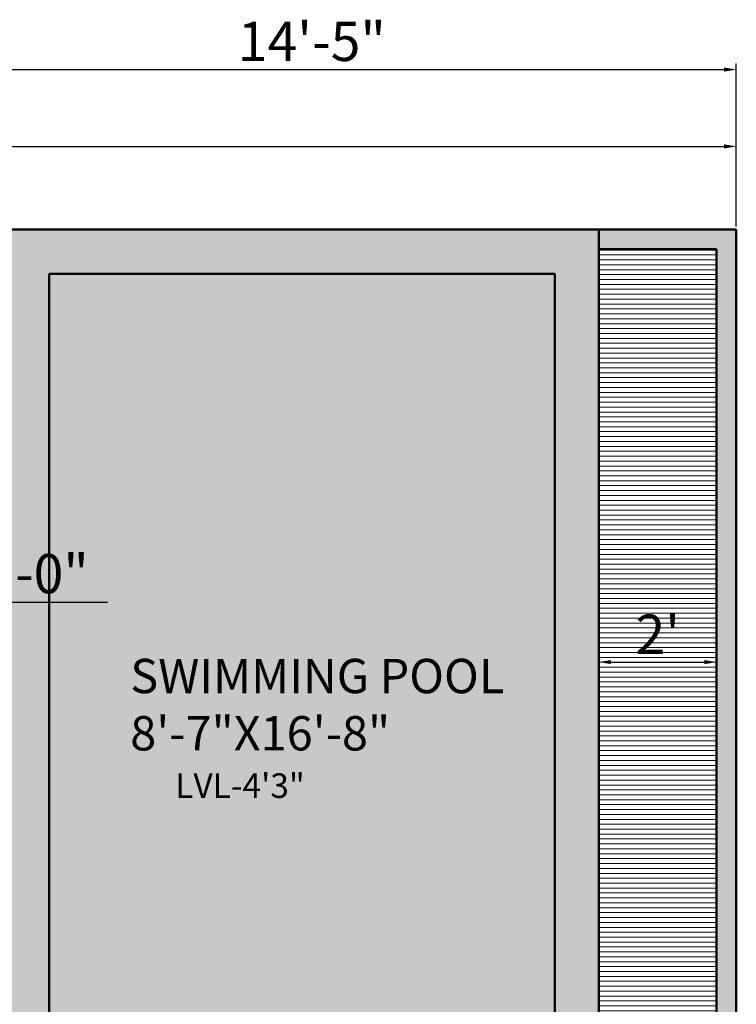
# Model space of a CAD drawing. Units: inches. Extents: x 1770 to 3141, y 984 to 1614.
# Tile 9 of 12: x 2267 to 2413, y 1407 to 1608. Entities that reach past the tile are written whole.
import ezdxf

# ---------------------------------------------------------------- set-up
doc = ezdxf.new("R2010")
doc.units = ezdxf.units.IN
for name, color, linetype, lineweight in [('A-ANNO-DIMS', 2, 'Continuous', 18), ('A-AREA-IDEN', 3, 'Continuous', 18), ('A-FLOR-PATT', 252, 'Continuous', 13), ('A-WALL', 7, 'Continuous', 50)]:
    doc.layers.add(name, color=color, linetype=linetype, lineweight=lineweight)
doc.styles.get("Standard").update_dxf_attribs({"font": 'arial.ttf'})
doc.dimstyles.new('ISO-25', dxfattribs={"dimtxt": 8, "dimasz": 2.5, "dimexe": 1.25, "dimexo": 0.625, "dimtad": 1, "dimdec": 1, "dimlunit": 3, "dimtxsty": 'Standard', "dimcen": 2.5, "dimclrt": 1, "dimadec": 0, "dimazin": 0, "dimtfac": 1, "dimtdec": 1, "dimtmove": 0, "dimatfit": 3, "dimfxl": 1, "dimarcsym": 0})

# ---------------------------------------------------------------- blocks, each defined once
blk = doc.blocks.new('*D17')
at = {"layer": 'A-ANNO-DIMS', "color": 0, "lineweight": -2, "transparency": 16777216}
for p, q in [((1812.73, 1565.8), (1812.73, 1583.37)), ((2412.73, 1565.8), (2412.73, 1583.37)), ((1815.23, 1582.12), (2410.23, 1582.12))]:
    blk.add_line(p, q, dxfattribs=at)
at = {"layer": 'A-ANNO-DIMS', "color": 0, "transparency": 16777216}
for points in [[(1815.23, 1582.54), (1815.23, 1581.7), (1812.73, 1582.12)], [(2410.23, 1582.54), (2410.23, 1581.7), (2412.73, 1582.12)]]:
    blk.add_solid(points, dxfattribs=at)
at = {"layer": 'Defpoints', "color": 0, "transparency": 16777216}
for p in [(2412.73, 1582.12), (1812.73, 1565.18), (2412.73, 1565.18)]:
    blk.add_point(p, dxfattribs=at)
at = {"layer": 'A-ANNO-DIMS', "color": 0, "transparency": 16777216, "insert": (2112.73, 1586.83), "char_height": 8, "attachment_point": 5}
blk.add_mtext("50'", dxfattribs=at)
blk = doc.blocks.new('*D64')
at = {"layer": 'A-ANNO-DIMS', "color": 0, "lineweight": -2, "transparency": 16777216}
for p, q in [((2384.73, 1477.67), (2384.73, 1478.3)), ((2387.23, 1477.05), (2406.23, 1477.05)), ((2408.73, 1477.67), (2408.73, 1478.3))]:
    blk.add_line(p, q, dxfattribs=at)
at = {"layer": 'A-ANNO-DIMS', "color": 0, "transparency": 16777216}
for points in [[(2387.23, 1477.46), (2387.23, 1476.63), (2384.73, 1477.05)], [(2406.23, 1477.46), (2406.23, 1476.63), (2408.73, 1477.05)]]:
    blk.add_solid(points, dxfattribs=at)
at = {"layer": 'Defpoints', "color": 0, "transparency": 16777216}
for p in [(2384.73, 1477.05), (2408.73, 1477.05), (2408.73, 1477.05)]:
    blk.add_point(p, dxfattribs=at)
at = {"layer": 'A-ANNO-DIMS', "color": 0, "transparency": 16777216, "insert": (2396.73, 1481.69), "char_height": 8, "attachment_point": 5}
blk.add_mtext("2'", dxfattribs=at)
blk = doc.blocks.new('*D90')
at = {"layer": 'A-ANNO-DIMS', "color": 0, "lineweight": -2, "transparency": 16777216}
for p, q in [((2148.77, 1492.24), (2148.77, 1488.01)), ((2172.77, 1492.24), (2172.77, 1488.01)), ((2151.27, 1489.26), (2170.27, 1489.26)), ((2172.77, 1489.26), (2284.63, 1489.26))]:
    blk.add_line(p, q, dxfattribs=at)
at = {"layer": 'A-ANNO-DIMS', "color": 0, "transparency": 16777216}
for points in [[(2151.27, 1489.68), (2151.27, 1488.84), (2148.77, 1489.26)], [(2170.27, 1489.68), (2170.27, 1488.84), (2172.77, 1489.26)]]:
    blk.add_solid(points, dxfattribs=at)
at = {"layer": 'Defpoints', "color": 0, "transparency": 16777216}
for p in [(2148.77, 1492.86), (2172.77, 1492.86), (2172.77, 1489.26)]:
    blk.add_point(p, dxfattribs=at)
at = {"layer": 'A-ANNO-DIMS', "color": 1, "transparency": 16777216, "insert": (2229.95, 1494.03), "char_height": 8, "attachment_point": 5}
blk.add_mtext('COFFEE TABLE 2\'-0"', dxfattribs=at)
blk = doc.blocks.new('*D104')
at = {"layer": 'A-ANNO-DIMS', "color": 0, "lineweight": -2, "transparency": 16777216}
for p, q in [((2239.73, 1565.8), (2239.73, 1599.03)), ((2412.73, 1565.8), (2412.73, 1599.03)), ((2242.23, 1597.78), (2410.23, 1597.78))]:
    blk.add_line(p, q, dxfattribs=at)
at = {"layer": 'A-ANNO-DIMS', "color": 0, "transparency": 16777216}
for points in [[(2242.23, 1598.2), (2242.23, 1597.36), (2239.73, 1597.78)], [(2410.23, 1598.2), (2410.23, 1597.36), (2412.73, 1597.78)]]:
    blk.add_solid(points, dxfattribs=at)
at = {"layer": 'Defpoints', "color": 0, "transparency": 16777216}
for p in [(2412.73, 1597.78), (2239.73, 1565.18), (2412.73, 1565.18)]:
    blk.add_point(p, dxfattribs=at)
at = {"layer": 'A-ANNO-DIMS', "color": 1, "transparency": 16777216, "insert": (2326.23, 1602.49), "char_height": 8, "attachment_point": 5}
blk.add_mtext('14\'-5"', dxfattribs=at)

msp = doc.modelspace()

# ---------------------------------------------------------------- hatches: boundary and pattern name
at = {"layer": 'A-FLOR-PATT'}
h = msp.add_hatch(color=256, dxfattribs=at)
h.dxf.hatch_style = 1
h.paths.add_polyline_path([(2263.73, 1565.18), (2239.73, 1565.18), (2239.73, 1561.18), (2263.73, 1561.18)])
h.paths.add_polyline_path([(2412.73, 1565.18), (2384.73, 1565.18), (2384.73, 1561.18), (2408.73, 1561.18), (2408.73, 1300.18), (2412.73, 1300.18)])
h = msp.add_hatch(color=256, dxfattribs=at)
h.dxf.hatch_style = 1
h.paths.add_polyline_path([(2384.73, 1565.18), (2263.73, 1565.18), (2263.73, 1347.18), (2333.73, 1347.18), (2333.73, 1356.18), (2272.73, 1356.18), (2272.73, 1556.18), (2375.73, 1556.18), (2375.73, 1347.18), (2384.73, 1347.18)])
h = msp.add_hatch(dxfattribs=at)
h.set_pattern_fill('_USER', color=256, pattern_type=0)
h.set_pattern_definition([(0, (0, 0), (0, 1), [])])
h.paths.add_polyline_path([(2408.73, 1561.18), (2384.73, 1561.18), (2384.73, 1347.18), (2375.73, 1347.18), (2263.73, 1347.18), (2263.73, 1561.18), (2239.73, 1561.18), (2239.73, 1300.18), (2408.73, 1300.18)])
h = msp.add_hatch(color=256, dxfattribs=at)
h.dxf.hatch_style = 1
h.paths.add_polyline_path([(2272.73, 1356.18), (2333.73, 1356.18), (2333.73, 1347.18), (2375.73, 1347.18), (2375.73, 1556.18), (2272.73, 1556.18)])
h.paths.add_polyline_path([(2287.05, 1445.97), (2372.59, 1445.97), (2372.59, 1481.19), (2287.05, 1481.19)], flags=24)

# ---------------------------------------------------------------- linework, layer by layer
at = {"layer": 'A-WALL'}
for p, q in [((1812.73, 1565.18), (2412.73, 1565.18)), ((2384.73, 1565.18), (2384.73, 1347.18)), ((2412.73, 1565.18), (2412.73, 1043.18)), ((2384.73, 1561.18), (2408.73, 1561.18)), ((2408.73, 1561.18), (2408.73, 1300.18)), ((2272.73, 1556.18), (2272.73, 1356.18)), ((2272.73, 1556.18), (2375.73, 1556.18)), ((2375.73, 1556.18), (2375.73, 1347.18))]:
    msp.add_line(p, q, dxfattribs=at)

# ---------------------------------------------------------------- texts
at = {"layer": 'A-AREA-IDEN', "insert": (2289.24, 1477.71), "char_height": 7, "attachment_point": 1}
msp.add_mtext_dynamic_manual_height_columns('SWIMMING POOL      8\'-7"X16\'-8"\\P{\\H0.71429x;      LVL-4\'3"}', width=86.9528, gutter_width=12.5, heights=[0], dxfattribs=at)

# ---------------------------------------------------------------- dimensions: what is measured, and where the dimension line sits
at = {"layer": 'A-ANNO-DIMS'}
for base, p1, p2, override, picture, middle in [((2412.73, 1597.78), (2239.73, 1565.18), (2412.73, 1565.18), {"dimdec": 1, "dimlfac": 1, "dimrnd": 0, "dimzin": 1, "dimdsep": 46, "dimlunit": 4, "dimfrac": 2}, '*D104', (2326.23, 1602.49)), ((2412.73, 1582.12), (1812.73, 1565.18), (2412.73, 1565.18), {"dimclrd": 0, "dimclre": 0, "dimclrt": 0}, '*D17', (2112.73, 1586.83)), ((2408.73, 1477.05), (2384.73, 1477.05), (2408.73, 1477.05), {"dimclrd": 0, "dimclre": 0, "dimclrt": 0}, '*D64', (2396.73, 1481.69))]:
    dim = msp.add_linear_dim(base=base, p1=p1, p2=p2, dimstyle='ISO-25', override=override, dxfattribs=at)
    dim.commit()
    dim.dimension.update_dxf_attribs({"geometry": picture, "text_midpoint": middle})
dim = msp.add_linear_dim(base=(2172.77, 1489.26), p1=(2148.77, 1492.86), p2=(2172.77, 1492.86), text='COFFEE TABLE <>', dimstyle='ISO-25', override={"dimdec": 1, "dimrnd": 0, "dimzin": 1, "dimlunit": 4, "dimfrac": 2}, dxfattribs=at)
dim.commit()
dim.dimension.update_dxf_attribs({"geometry": '*D90', "text_midpoint": (2229.95, 1494.03)})

doc.saveas('drawing.dxf')
